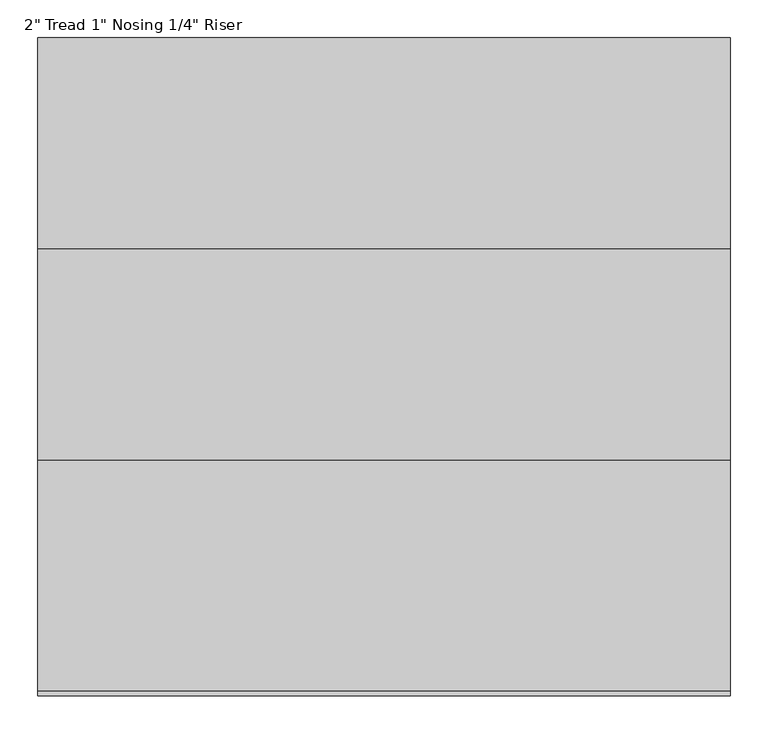
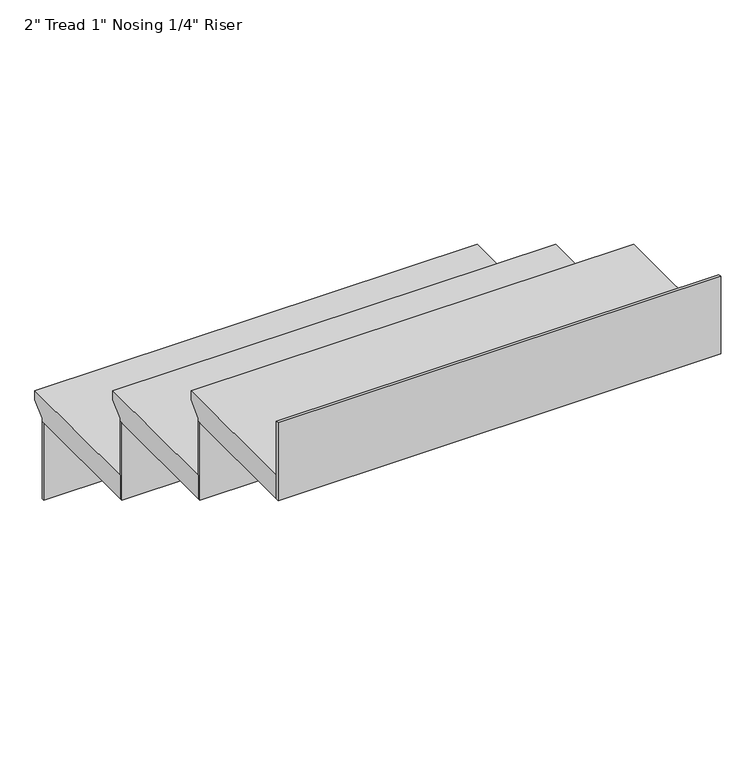
"""IFC4 building model written with IfcOpenShell, lengths in millimetres: stair flight geometry."""

from ifc_helpers import new_model, si_unit, frame, origin, place, context, project, spatial, polyline, outline, extrude, source, transform, mapped, element, save


def stair_flight_f3376f64(model_context):
    return source(origin(), model_context, "Body", "SweptSolid", [
        extrude(outline(polyline([(-19826.9851539, 39966.6172466), (-19522.1851539, 39966.6172466), (-19522.1851539, 39947.5672466), (-19547.5851539, 39922.1672466), (-19547.5851539, 39915.8172466), (-19826.9851539, 39915.8172466), (-19826.9851539, 39966.6172466)])), frame((-2296.6415084, 0.0, 0.0), z_axis=(1.0, 0.0, 0.0), x_axis=(0.0, 1.0, 0.0)), (0.0, 0.0, 1.0), 914.4),
        extrude(outline(polyline([(-2296.6415084, -19553.9351539), (-2296.6415084, -19547.5851539), (-1382.2415084, -19547.5851539), (-1382.2415084, -19553.9351539), (-2296.6415084, -19553.9351539)])), frame((0.0, 0.0, 39746.4839133), z_axis=(0.0, 0.0, 1.0), x_axis=(1.0, 0.0, 0.0)), (0.0, 0.0, 1.0), 169.3333333),
        extrude(outline(polyline([(-2296.6415084, -19833.3351539), (-2296.6415084, -19826.9851539), (-1382.2415084, -19826.9851539), (-1382.2415084, -19833.3351539), (-2296.6415084, -19833.3351539)])), frame((0.0, 0.0, 39915.8172466), z_axis=(0.0, 0.0, 1.0), x_axis=(1.0, 0.0, 0.0)), (0.0, 0.0, 1.0), 169.3333333),
        extrude(outline(polyline([(-20106.3851539, 40135.9505799), (-19801.5851539, 40135.9505799), (-19801.5851539, 40116.9005799), (-19826.9851539, 40091.5005799), (-19826.9851539, 40085.1505799), (-20106.3851539, 40085.1505799), (-20106.3851539, 40135.9505799)])), frame((-2296.6415084, 0.0, 0.0), z_axis=(1.0, 0.0, 0.0), x_axis=(0.0, 1.0, 0.0)), (0.0, 0.0, 1.0), 914.4),
        extrude(outline(polyline([(-2296.6415084, -20112.7351539), (-2296.6415084, -20106.3851539), (-1382.2415084, -20106.3851539), (-1382.2415084, -20112.7351539), (-2296.6415084, -20112.7351539)])), frame((0.0, 0.0, 40085.1505799), z_axis=(0.0, 0.0, 1.0), x_axis=(1.0, 0.0, 0.0)), (0.0, 0.0, 1.0), 169.3333333),
        extrude(outline(polyline([(-2296.6415084, -20392.1351539), (-2296.6415084, -20385.7851539), (-1382.2415084, -20385.7851539), (-1382.2415084, -20392.1351539), (-2296.6415084, -20392.1351539)])), frame((0.0, 0.0, 40254.4839133), z_axis=(0.0, 0.0, 1.0), x_axis=(1.0, 0.0, 0.0)), (0.0, 0.0, 1.0), 169.3333333),
        extrude(outline(polyline([(-20385.7851539, 40305.2839133), (-20080.9851539, 40305.2839133), (-20080.9851539, 40286.2339133), (-20106.3851539, 40260.8339133), (-20106.3851539, 40254.4839133), (-20385.7851539, 40254.4839133), (-20385.7851539, 40305.2839133)])), frame((-2296.6415084, 0.0, 0.0), z_axis=(1.0, 0.0, 0.0), x_axis=(0.0, 1.0, 0.0)), (0.0, 0.0, 1.0), 914.4),
    ])


if __name__ == "__main__":
    model = new_model("IFC4")
    model_context = context("Model", 3, world=origin())
    ifc_project = project(units=[si_unit("LENGTHUNIT", "METRE", prefix="MILLI")], contexts=[model_context])
    site = spatial("IfcSite", under=ifc_project)
    building = spatial("IfcBuilding", under=site)
    placement = place(None, origin())
    stair_flight_shape = stair_flight_f3376f64(model_context)
    element("IfcStairFlight", 1, ObjectType="2\" Tread 1\" Nosing 1/4\" Riser", at=placement, inside=building, context=model_context, shape_type="MappedRepresentation", body=[
        mapped(stair_flight_shape, transform((0.0, 0.0, 0.0), x_axis=(1.0, 0.0, 0.0), y_axis=(0.0, 1.0, 0.0), z_axis=(0.0, 0.0, 1.0))),
    ])
    save(model, "model.ifc")
